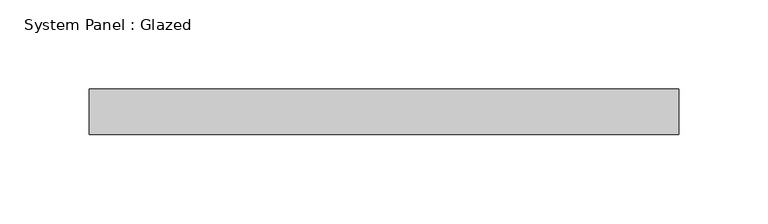
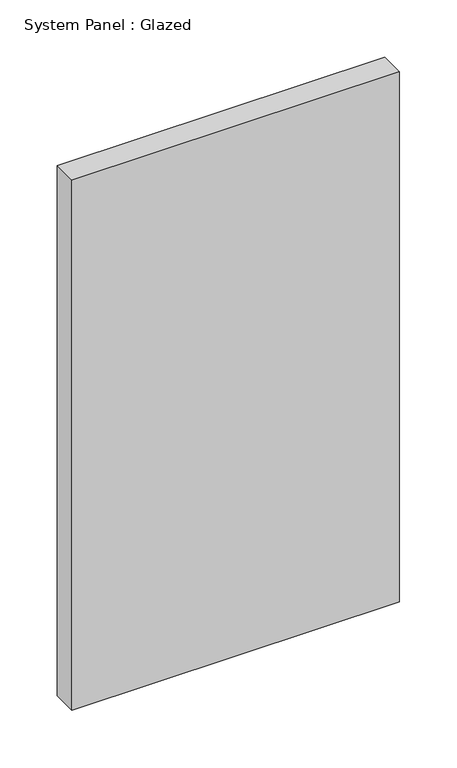
"""IFC4 building model written with IfcOpenShell, lengths in millimetres: plate geometry, System Panel : Glazed."""

from ifc_helpers import new_model, si_unit, origin, origin_with_axes, place, context, project, spatial, polyline, outline, extrude, source, transform, mapped, element, save


def system_panel_glazed_997bcd70(model_context):
    return source(origin(), model_context, "Body", "SweptSolid", [
        extrude(outline(polyline([(165.1, 19.05), (-165.1, 19.05), (-165.1, 44.45), (165.1, 44.45), (165.1, 19.05)])), origin_with_axes(), (0.0, 0.0, 1.0), 565.2549172),
    ])


if __name__ == "__main__":
    model = new_model("IFC4")
    model_context = context("Model", 3, world=origin())
    ifc_project = project(units=[si_unit("LENGTHUNIT", "METRE", prefix="MILLI")], contexts=[model_context])
    site = spatial("IfcSite", under=ifc_project)
    building = spatial("IfcBuilding", under=site)
    placement = place(None, origin())
    system_panel_glazed_shape = system_panel_glazed_997bcd70(model_context)
    element("IfcPlate", 1, ObjectType="System Panel : Glazed", at=placement, inside=building, context=model_context, shape_type="MappedRepresentation", body=[
        mapped(system_panel_glazed_shape, transform((0.0, 0.0, 0.0), x_axis=(1.0, 0.0, 0.0), y_axis=(0.0, 1.0, 0.0), z_axis=(0.0, 0.0, 1.0))),
    ])
    save(model, "model.ifc")

# Revit data of these elements
# Type "System Panel : Glazed"
#   Construction Type Id = "GSP4R"
#   Analytic Construction = "1/8 in Pilkington single glazing"
#   Visual Light Transmittance = 0.9
#   Solar Heat Gain Coefficient = 0.86
#   Heat Transfer Coefficient (U) = 1.18115 BTU/(h·ft²·°F)
#   Define Thermal Properties by = 1
# Element 1 (IfcPlate, "System Panel : Glazed")
#   Materials on its faces: "Glass"
# Materials
#   "Glass": class "Glass", colour RGB 0 128 192, transparency 0.75, Description = "Soda Lime Glass", Cost = 0
